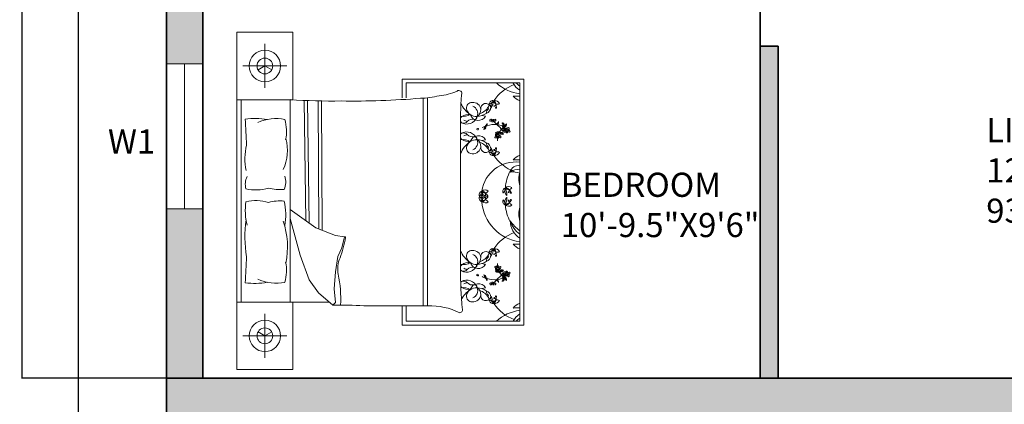
# Model space of a CAD drawing. Units: inches. Extents: x -9 to 505, y -680 to 48.
# Tile 3 of 17: x -9 to 235, y -293 to -198. Entities that reach past the tile are written whole.
import ezdxf

# ---------------------------------------------------------------- set-up
doc = ezdxf.new("R2010")
doc.units = ezdxf.units.IN
doc.header["$MEASUREMENT"] = 0
for name, color, linetype, lineweight in [('A-ANNO-DIMS', 2, 'Continuous', 18), ('A-ANNO-TEXT', 7, 'Continuous', 18), ('A-AREA-IDEN', 7, 'Continuous', 18), ('A-FURN', 8, 'Continuous', 18), ('A-GLAZ', 4, 'Continuous', 18), ('A-WALL', 7, 'Continuous', 35), ('A-WALL-PATT', 251, 'Continuous', 13), ('S-CONC', 7, 'Continuous', 35), ('S-CONC-PATT', 18, 'Continuous', 13)]:
    doc.layers.add(name, color=color, linetype=linetype, lineweight=lineweight)
doc.styles.get("Standard").update_dxf_attribs({"font": 'arial.ttf'})
doc.dimstyles.get("Standard").update_dxf_attribs({"dimtxt": 0.18, "dimasz": 0.18, "dimexe": 0.18, "dimexo": 0.0625, "dimgap": 0.09, "dimtad": 0, "dimtih": 1, "dimtoh": 1, "dimdec": 0, "dimzin": 0, "dimdsep": 46, "dimlunit": 3, "dimtxsty": 'Standard', "dimcen": 0.09, "dimadec": 0, "dimazin": 0, "dimtfac": 1, "dimtdec": 0, "dimtofl": 0, "dimtmove": 0, "dimatfit": 3, "dimfxl": 1, "dimtolj": 1, "dimtzin": 0, "dimarcsym": 0})

# ---------------------------------------------------------------- blocks, each defined once
blk = doc.blocks.new('*D3')
at = {"layer": 'A-ANNO-DIMS', "color": 0, "lineweight": -2, "transparency": 16777216}
for p, q in [((27.2, 11.5), (5.16, 11.5)), ((5.34, 11.32), (5.34, -330.86)), ((5.34, -679.32), (5.34, -337.14)), ((27.2, -679.5), (5.16, -679.5))]:
    blk.add_line(p, q, dxfattribs=at)
at = {"layer": 'A-ANNO-DIMS', "color": 0, "transparency": 16777216}
for points in [[(5.31, 11.32), (5.37, 11.32), (5.34, 11.5)], [(5.31, -679.32), (5.37, -679.32), (5.34, -679.5)]]:
    blk.add_solid(points, dxfattribs=at)
at = {"layer": 'Defpoints', "color": 0, "transparency": 16777216}
for p in [(27.26, 11.5), (5.34, -679.5), (27.26, -679.5)]:
    blk.add_point(p, dxfattribs=at)
at = {"layer": 'A-ANNO-DIMS', "color": 0, "transparency": 16777216, "insert": (5.34, -334), "char_height": 6, "attachment_point": 5}
blk.add_mtext('\\A1;57\'-7"', dxfattribs=at)
blk = doc.blocks.new('WIN-36')
for p, q in [((0, 36), (0, 0)), ((9, 36), (0, 36)), ((4.5, 36), (4.5, 2.23)), ((9, 0), (9, 36)), ((0, 0), (9, 0)), ((4.5, 2.23), (4.5, 0))]:
    blk.add_line(p, q)
blk = doc.blocks.new('*D46')
at = {"layer": 'A-ANNO-DIMS', "color": 0, "lineweight": -2, "transparency": 16777216}
for p, q in [((27.2, 11.5), (-8.8, 11.5)), ((-8.62, 11.32), (-8.62, -137.57)), ((-8.62, -286.82), (-8.62, -137.93)), ((27.2, -287), (-8.8, -287))]:
    blk.add_line(p, q, dxfattribs=at)
at = {"layer": 'A-ANNO-DIMS', "color": 0, "transparency": 16777216}
for points in [[(-8.65, 11.32), (-8.59, 11.32), (-8.62, 11.5)], [(-8.65, -286.82), (-8.59, -286.82), (-8.62, -287)]]:
    blk.add_solid(points, dxfattribs=at)
at = {"layer": 'Defpoints', "color": 0, "transparency": 16777216}
for p in [(27.26, 11.5), (-8.62, -287), (27.26, -287)]:
    blk.add_point(p, dxfattribs=at)
at = {"layer": 'A-ANNO-DIMS', "color": 0, "transparency": 16777216, "insert": (-8.62, -137.75), "char_height": 0.18, "attachment_point": 5}
blk.add_mtext('\\A1;24\'-10 1/2"', dxfattribs=at)

msp = doc.modelspace()

# ---------------------------------------------------------------- hatches: boundary and pattern name
at = {"layer": 'A-WALL-PATT'}
h = msp.add_hatch(color=256, dxfattribs=at)
h.dxf.hatch_style = 1
h.paths.add_polyline_path([(101.64, 11.5), (48.26, 11.5), (48.26, 2.5), (72.26, 2.5), (72.26, -21.25), (81.26, -21.25), (81.26, 2.5), (101.64, 2.5)])
h.paths.add_polyline_path([(36.26, 2.5), (27.26, 2.5), (27.26, -6.92), (36.26, -6.92)])
h.paths.add_polyline_path([(81.26, -57.25), (72.26, -57.25), (72.26, -75.5), (81.26, -75.5)])
h.paths.add_polyline_path([(162.76, 11.5), (137.64, 11.5), (137.64, 2.5), (162.76, 2.5)])
h.paths.add_polyline_path([(179.26, 2.5), (174.76, 2.5), (174.76, -75.5), (179.26, -75.5), (179.26, -54.5), (229.51, -54.5), (229.51, -45.5), (179.26, -45.5)])
h.paths.add_polyline_path([(382.26, -45.5), (332.26, -45.5), (332.26, 2.5), (327.76, 2.5), (327.76, -45.5), (277.51, -45.5), (277.51, -54.5), (327.76, -54.5), (327.76, -111.5), (332.26, -111.5), (332.26, -54.5), (382.26, -54.5)])
h.paths.add_polyline_path([(332.26, -128), (327.76, -128), (327.76, -207), (332.26, -207)])
h.paths.add_polyline_path([(124.76, -111.5), (36.26, -111.5), (36.26, -116), (120.26, -116), (120.26, -168.5), (179.26, -168.5), (179.26, -164), (124.76, -164)])
h.paths.add_polyline_path([(96.26, -164), (36.26, -164), (36.26, -152), (27.26, -152), (27.26, -208.88), (36.26, -208.88), (36.26, -168.5), (96.26, -168.5)])
h.paths.add_polyline_path([(36.26, -244.88), (27.26, -244.88), (27.26, -287), (36.26, -287)])
h.paths.add_polyline_path([(179.26, -204.5), (174.76, -204.5), (174.76, -287), (179.26, -287)])
h.paths.add_polyline_path([(257.26, -296), (248.26, -296), (248.26, -446), (269.26, -446), (269.26, -437), (257.26, -437)])
h.paths.add_polyline_path([(90.26, -296), (81.26, -296), (81.26, -348.67), (90.26, -348.67)])
h.paths.add_polyline_path([(90.26, -384.67), (81.26, -384.67), (81.26, -416), (90.26, -416)])
h.paths.add_polyline_path([(170.26, -452), (36.26, -452), (36.26, -456.5), (165.76, -456.5), (165.76, -504.5), (165.13, -504.5), (165.13, -509), (170.26, -509)])
h.paths.add_polyline_path([(141.76, -504.5), (36.26, -504.5), (36.26, -492.5), (27.26, -492.5), (27.26, -565.96), (36.26, -565.96), (36.26, -509), (141.76, -509)])
h.paths.add_polyline_path([(36.26, -601.96), (27.26, -601.96), (27.26, -658.5), (36.26, -658.5)])
h.paths.add_polyline_path([(170.26, -670.5), (170.26, -634.5), (222.76, -634.5), (222.76, -625.5), (165.76, -625.5), (165.76, -670.5), (36.26, -670.5), (36.26, -679.5), (170.26, -679.5)])
h.paths.add_polyline_path([(332.26, -616.5), (433.89, -616.5), (433.89, -612), (332.26, -612), (332.26, -610.56), (327.76, -610.56), (327.76, -625.5), (270.76, -625.5), (270.76, -634.5), (327.76, -634.5), (327.76, -658.5), (332.26, -658.5)])
h.paths.add_polyline_path([(459.76, -670.5), (336.76, -670.5), (336.76, -679.5), (459.76, -679.5)])
h.paths.add_polyline_path([(468.76, -545.74), (459.76, -545.74), (459.76, -612), (457.89, -612), (457.89, -616.5), (459.76, -616.5), (459.76, -658.5), (468.76, -658.5)])
h.paths.add_polyline_path([(332.26, -446), (327.76, -446), (327.76, -574.56), (332.26, -574.56)])
h.paths.add_polyline_path([(327.76, -437), (305.26, -437), (305.26, -446), (327.76, -446)])
h.paths.add_polyline_path([(459.76, -437), (348.76, -437), (348.76, -446), (459.76, -446)])
h.paths.add_polyline_path([(468.76, -458), (459.76, -458), (459.76, -509.74), (468.76, -509.74)])
h.paths.add_polyline_path([(468.76, -365), (459.76, -365), (459.76, -437), (468.76, -437)])
h.paths.add_polyline_path([(468.76, -299.6), (459.76, -299.6), (459.76, -344), (468.76, -344)])
h.paths.add_polyline_path([(468.76, -184.74), (459.76, -184.74), (459.76, -231), (401.26, -231), (401.26, -235.5), (459.76, -235.5), (459.76, -275.6), (468.76, -275.6)])
h.paths.add_polyline_path([(390.76, -356), (342.76, -356), (342.76, -365), (390.76, -365)])
h.paths.add_polyline_path([(459.76, -356), (405.76, -356), (405.76, -365), (459.76, -365)])
h.paths.add_polyline_path([(405.76, -296), (396.76, -296), (396.76, -356), (405.76, -356)])
h.paths.add_polyline_path([(336.76, -296), (327.76, -296), (327.76, -356), (336.76, -356)])
h.paths.add_polyline_path([(468.76, -9.5), (459.76, -9.5), (459.76, -45.5), (418.26, -45.5), (418.26, -54.5), (468.76, -54.5)])
h.paths.add_polyline_path([(468.76, -54.5), (459.76, -54.5), (459.76, -111.5), (468.76, -111.5)])
h.paths.add_polyline_path([(468.76, -128), (459.76, -128), (459.76, -148.74), (468.76, -148.74)])
at = {"layer": 'S-CONC-PATT'}
h = msp.add_hatch(color=256, dxfattribs=at)
h.dxf.hatch_style = 1
h.paths.add_polyline_path([(269.26, -296), (269.26, -287), (27.26, -287), (27.26, -308), (36.26, -308), (36.26, -296)])

# ---------------------------------------------------------------- linework, layer by layer
at = {"layer": 'A-FURN'}
for p, q in [((44.71, -284.86), (44.71, -201.01)), ((51.7, -214.87), (51.7, -203.92)), ((57.17, -209.4), (46.22, -209.4)), ((85.81, -217.31), (85.81, -212.66)), ((85.81, -212.66), (116.01, -212.66)), ((116.01, -212.66), (116.01, -273.79)), ((86.78, -213.63), (86.78, -217.33)), ((115.04, -213.63), (86.78, -213.63)), ((115.04, -272.82), (115.04, -213.63)), ((91.04, -217.4), (91.04, -269.05)), ((92.08, -217.32), (92.08, -269.05)), ((45.78, -217.78), (45.78, -268.09)), ((57.96, -268.09), (57.96, -217.78)), ((61.44, -218.01), (61.86, -247.86)), ((62.3, -218.04), (62.73, -248.48)), ((64.94, -218.08), (65.07, -249.92)), ((65.8, -218.08), (65.93, -250.25)), ((106.54, -221.9), (105.59, -221.71)), ((100.32, -225.91), (100.32, -259.95)), ((106.54, -227.76), (105.59, -227.94)), ((57.96, -245.05), (64.35, -249.65)), ((60.45, -256.44), (57.96, -247.3)), ((64.35, -249.65), (69.28, -251.52)), ((69.28, -251.52), (71.48, -251.86)), ((71.48, -251.86), (70.8, -254.57)), ((62.66, -262.55), (60.45, -256.44)), ((69.78, -256.78), (69.28, -260.52)), ((70.8, -254.57), (69.78, -256.78)), ((106.54, -258.7), (105.59, -258.51)), ((69.28, -260.52), (68.94, -264.76)), ((65.03, -265.78), (62.66, -262.55)), ((68.6, -268.84), (65.03, -265.78)), ((68.94, -264.76), (69.28, -268.16)), ((106.54, -264.56), (105.59, -264.74)), ((44.71, -268.09), (67.72, -268.09)), ((69.28, -268.16), (68.6, -268.84)), ((85.81, -273.79), (85.81, -269.05)), ((86.78, -269.05), (86.78, -272.82)), ((51.7, -270.99), (51.7, -281.95)), ((116.01, -273.79), (85.81, -273.79)), ((86.78, -272.82), (115.04, -272.82)), ((57.17, -276.47), (46.22, -276.47))]:
    msp.add_line(p, q, dxfattribs=at)
for points in [[(44.71, -217.78), (58.68, -217.78), (58.68, -201.01), (44.71, -201.01)], [(51.7, -209.4), (50, -210.37)], [(51.7, -209.4), (53.39, -210.37)], [(58.68, -268.09), (58.68, -284.86), (44.71, -284.86)], [(51.7, -276.47), (50, -275.49)], [(51.7, -276.47), (53.39, -275.49)]]:
    msp.add_lwpolyline(points, dxfattribs=at)
for points in [[(90.38, -217.42, 0.056112), (94.99, -216.81, 0.095341), (99.43, -215.64)], [(46.8, -222.6, -0.074897), (52.27, -222.7, 0.472817)], [(52.58, -239.75, -0.14099), (46.99, -239.91, -0.235245)], [(52.58, -243.33, 0.14099), (46.99, -243.16, 0.235245)], [(46.8, -263.27, 0.074897), (52.27, -263.17, -0.472817)], [(76.27, -269.01, 0.001242), (92.18, -269.05, -0.127202), (100.11, -270.73)]]:
    msp.add_lwpolyline(points, format="xyb", dxfattribs=at)
for centre, radius in [((51.7, -209.4), 3.91), ((51.7, -209.4), 1.96), ((109.58, -226.74), 0.214), ((111.83, -225.34), 0.214), ((109.58, -259.71), 0.214), ((111.83, -261.11), 0.214), ((51.7, -276.47), 3.91), ((51.7, -276.47), 1.96)]:
    msp.add_circle(centre, radius, dxfattribs=at)
for centre, radius, start, end in [((117.6, -224.22), 10.95, 111.4092, 145.6135), ((116.52, -205.48), 10.95, 228.1144, 262.255), ((117.98, -210.98), 5.34, 209.8884, 236.5383), ((118.98, -209.06), 6.65, 223.5186, 233.6964), ((73.68, -21.61), 196.52, 269.1145, 274.8735), ((99.86, -216.27), 0.764, 336.5219, 123.8264), ((181.87, -223.34), 81.59, 175.2402, 181.8035), ((116.75, -213.96), 4.45, 221.0454, 247.4453), ((114.36, -201.77), 15.15, 266.3481, 272.5919), ((68.2, -67.47), 150.65, 266.1, 270.9282), ((106.22, -216.16), 6.35, 203.6453, 236.3329), ((103.18, -219.86), 1.42, 88.9462, 185.5144), ((104.22, -219.43), 2.52, 193.079, 274.7067), ((103.38, -220.44), 2, 7.1143, 95.0551), ((102.62, -221.23), 1.95, 338.5779, 68.4181), ((103.84, -217.48), 3.96, 288.2955, 328.7386), ((106.61, -219.98), 1.26, 19.1312, 189.736), ((106.23, -219.68), 1.57, 285.6955, 4.031), ((108.32, -221.37), 1.67, 128.4175, 173.8338), ((107.97, -219.72), 0.771, 126.7319, 206.0245), ((108.35, -218.91), 0.908, 76.272, 177.0484), ((106.97, -217.06), 1.87, 284.7031, 328.6173), ((109.57, -219.44), 1.73, 125.7657, 194.5347), ((101.09, -216.37), 7.66, 332.8176, 347.4827), ((108.82, -219.22), 1.21, 20.9613, 102.2885), ((109.48, -218), 0.914, 181.7131, 301.5367), ((106.48, -219.85), 2.77, 2.0648, 41.1598), ((108.15, -218.82), 0.896, 316.2238, 62.3173), ((108.66, -219.35), 0.0714, 20.2667, 316.2271), ((109.11, -219.76), 0.136, 168.5166, 2.0648), ((109.04, -219.75), 0.0661, 52.0591, 168.5166), ((-751.12, -268.81), 799.26, 2.85022, 3.31479), ((54.47, -233.28), 10.81, 78.2417, 114.8684), ((101.25, -222.79), 1.01, 127.675, 162.5814), ((100.94, -218.49), 3.47, 259.249, 301.1782), ((101.84, -221.18), 2.67, 240.8249, 340.7178), ((102.45, -224.67), 3.23, 85.2696, 124.215), ((103.27, -224.34), 1.72, 74.8529, 138.4347), ((104.73, -220.86), 2.08, 196.8663, 330.0915), ((103.86, -222.18), 0.52, 254.8529, 12.6959), ((102.45, -224.67), 3.23, 53.6555, 57.2989), ((102.93, -220.09), 2.44, 305.9599, 357.6409), ((104.16, -217.45), 4.5, 273.4924, 303.7117), ((107.98, -222.9), 0.356, 127.3642, 168.4363), ((108.31, -222.6), 0.214, 183.2768, 356.7232), ((108.7, -222.89), 0.353, 10.9597, 52.2379), ((45.82, -225.59), 11.24, 348.9631, 14.8961), ((101.25, -222.79), 1.01, 196.6343, 225.5483), ((101.05, -222.37), 1.25, 246.1646, 318.4347), ((102.33, -220.78), 2.41, 240.0851, 262.564), ((104.55, -225.05), 0.263, 169.5864, 349.5616), ((104.65, -225.07), 0.162, 349.5616, 167.2949), ((108.87, -230.88), 6.94, 110.1059, 116.9968), ((105.27, -224.14), 1.33, 308.4388, 328.836), ((106.54, -225.16), 0.44, 129.5056, 182.6421), ((105.04, -223.06), 2.36, 296.5064, 305.3102), ((105.02, -224.28), 1.35, 336.3901, 344.4871), ((106.49, -224.62), 0.171, 83.9457, 185.6216), ((105.81, -224.46), 0.703, 328.836, 0.8141), ((106.17, -224.67), 0.402, 306.5232, 32.4668), ((106.65, -224.35), 0.171, 112.5583, 214.2343), ((106.54, -224.05), 0.402, 265.7131, 351.6568), ((106.19, -223.83), 0.703, 297.3659, 329.344), ((105.65, -223.22), 1.35, 313.6929, 321.7899), ((107.14, -224.14), 0.44, 115.5379, 168.6744), ((105.65, -223.51), 1.33, 329.344, 349.7412), ((108.87, -230.88), 6.94, 86.1723, 106.4158), ((104.59, -223.81), 2.36, 352.8698, 1.6736), ((107.72, -222.96), 0.165, 125.0752, 284.7644), ((107.7, -222.61), 0.513, 277.4968, 341.2737), ((108.11, -222.85), 0.204, 88.1325, 178.8919), ((108.52, -223.07), 0.441, 136.3462, 189.6513), ((108.26, -223.11), 0.184, 189.6513, 312.3208), ((108.98, -222.98), 0.699, 164.2829, 186.9148), ((108.15, -222.99), 0.349, 312.3208, 40.2111), ((108.89, -222.59), 0.496, 201.6382, 274.947), ((108.24, -223.27), 0.648, 42.3896, 66.5724), ((114.78, -218.14), 7.96, 217.9541, 226.8459), ((108.92, -222.93), 0.164, 274.947, 37.5263), ((109.47, -223.85), 0.171, 112.5583, 214.2343), ((109.36, -223.55), 0.402, 265.7131, 351.6568), ((109.01, -223.33), 0.703, 297.3659, 329.344), ((109.04, -227.42), 3.48, 60.7959, 85.244), ((101.63, -232.43), 11.46, 37.8256, 47.7588), ((108.48, -222.72), 1.35, 313.6929, 321.7899), ((109.97, -223.64), 0.44, 115.5379, 168.6744), ((108.47, -223.01), 1.33, 329.344, 349.7412), ((107.41, -223.31), 2.36, 352.8698, 1.6736), ((113.67, -227.78), 4.18, 130.182, 149.456), ((110.74, -223.79), 0.238, 33.0979, 123.1364), ((105.49, -227.15), 6.24, 31.1156, 34.8118), ((110.39, -224.2), 0.645, 2.3172, 70.5201), ((111.37, -225.4), 0.689, 139.3812, 199.9959), ((110.08, -224.9), 0.973, 310.9365, 22.7695), ((110.93, -224.36), 0.186, 135.7354, 318.1297), ((110.61, -224.06), 0.247, 315.7354, 31.1156), ((110.41, -224.58), 0.573, 319.3812, 5.5456), ((111.06, -224.36), 0.186, 68.2452, 250.6395), ((110.64, -224.13), 0.556, 352.6008, 57.1845), ((112.62, -227.86), 3.72, 111.7087, 116.2181), ((109.04, -227.42), 3.48, 47.5083, 55.9967), ((111.17, -224), 0.556, 252.8042, 349.6943), ((110.64, -225), 0.592, 331.1838, 51.6792), ((111.23, -223.96), 0.247, 248.2452, 323.6254), ((111.45, -225.08), 0.209, 138.2946, 276.2474), ((111.01, -223.8), 0.645, 291.7087, 3.0299), ((111.53, -225.11), 0.291, 358.5719, 143.8954), ((106.4, -220.4), 6.24, 323.6254, 327.3216), ((111.7, -224.88), 0.294, 208.8493, 269.9355), ((111.52, -223.97), 0.238, 325.6077, 55.6462), ((112.47, -225.29), 0.673, 121.9501, 165.2442), ((112.01, -225.03), 0.141, 262.868, 7.094), ((111.99, -224.91), 0.421, 278.5614, 22.5914), ((112.23, -224.9), 0.212, 44.3732, 121.9501), ((46.64, -230.44), 10.67, 333.8761, 16.1746), ((101.25, -226.86), 1.01, 134.4517, 156.7144), ((101.25, -226.86), 1.01, 203.2856, 232.325), ((101.84, -228.47), 2.67, 19.2822, 119.1751), ((101.05, -227.29), 1.25, 41.5653, 113.8354), ((102.33, -228.88), 2.41, 97.436, 119.9149), ((103.27, -225.31), 1.72, 221.5653, 285.1471), ((104.73, -228.8), 2.08, 29.9085, 163.1337), ((103.86, -227.48), 0.52, 347.3041, 105.1471), ((108.99, -227.1), 0.165, 125.0752, 284.7644), ((109.25, -227.04), 0.356, 93.635, 168.4363), ((109.26, -225.11), 0.973, 253.6301, 325.4631), ((109.53, -226.46), 0.689, 82.0748, 142.6895), ((109.46, -225.51), 0.707, 228.342, 274.9894), ((109.2, -226.47), 0.209, 138.2946, 276.2474), ((108.97, -226.75), 0.513, 277.4968, 341.2737), ((109.28, -226.51), 0.291, 358.5719, 143.8954), ((109.38, -226.99), 0.204, 88.1325, 178.8919), ((109.45, -226.28), 0.294, 208.8493, 269.9355), ((109.2, -226.35), 0.336, 274.2123, 318.1587), ((109.79, -227.21), 0.441, 136.3462, 189.6513), ((109.53, -227.25), 0.184, 189.6513, 312.3208), ((113.67, -227.78), 4.18, 175.2415, 182.8929), ((109.48, -225.63), 0.592, 273.8774, 357.1501), ((110.25, -227.12), 0.699, 164.2829, 186.9148), ((110.22, -226.68), 0.673, 121.9501, 165.2442), ((109.71, -225.21), 0.573, 262.0748, 308.2393), ((109.42, -227.13), 0.349, 312.3208, 40.2111), ((110.16, -226.73), 0.496, 201.6382, 274.947), ((109.76, -226.42), 0.141, 262.868, 7.094), ((109.5, -227.41), 0.648, 42.3896, 66.5724), ((109.74, -226.31), 0.421, 278.5614, 22.5914), ((109.97, -227.03), 0.353, 10.9597, 118.7804), ((113.67, -227.78), 4.18, 156.1523, 156.9499), ((109.98, -226.29), 0.212, 44.3732, 121.9501), ((110.63, -225.79), 0.592, 181.4625, 249.4747), ((110.53, -225.33), 0.573, 215.1128, 261.2773), ((110.99, -225.36), 0.973, 197.889, 269.722), ((110.19, -227.06), 0.164, 274.947, 37.5263), ((110.69, -225.69), 0.707, 248.3627, 295.0101), ((110.34, -226.58), 0.689, 20.6625, 81.2773), ((110.53, -224.95), 0.707, 285.6484, 332.2957), ((111.24, -225.7), 0.165, 125.0752, 284.7644), ((111.5, -225.64), 0.356, 93.635, 168.4363), ((111.22, -225.35), 0.513, 277.4968, 341.2737), ((111.63, -225.59), 0.204, 88.1325, 178.8919), ((111.45, -224.95), 0.336, 274.2123, 318.1587), ((112.04, -225.81), 0.441, 136.3462, 189.6513), ((111.78, -225.85), 0.184, 189.6513, 312.3208), ((112.5, -225.73), 0.699, 164.2829, 186.9148), ((111.67, -225.73), 0.349, 312.3208, 40.2111), ((112.41, -225.34), 0.496, 201.6382, 274.947), ((111.75, -226.02), 0.648, 42.3896, 66.5724), ((112.22, -225.64), 0.353, 10.9597, 118.7804), ((112.44, -225.67), 0.164, 274.947, 37.5263), ((61.47, -232.55), 14.74, 166.3427, 191.1841), ((100.94, -231.16), 3.47, 58.8218, 100.2867), ((106.22, -233.49), 6.35, 123.6671, 158.5059), ((102.45, -224.99), 3.23, 235.785, 274.7304), ((103.18, -229.79), 1.42, 174.4856, 271.0538), ((104.22, -230.23), 2.52, 85.2933, 166.921), ((103.38, -229.21), 2, 264.9449, 352.8857), ((102.62, -228.43), 1.95, 291.5819, 21.4221), ((102.45, -224.99), 3.23, 302.7011, 306.3445), ((102.93, -229.56), 2.44, 2.3591, 54.0401), ((104.16, -232.21), 4.5, 56.2883, 86.5076), ((103.84, -232.17), 3.96, 31.2614, 71.7045), ((106.61, -229.67), 1.26, 170.264, 340.8688), ((108.32, -228.28), 1.67, 186.1662, 231.5825), ((106.23, -229.98), 1.57, 355.969, 74.3045), ((107.97, -229.93), 0.771, 153.9755, 233.2681), ((109.57, -230.22), 1.73, 165.4653, 234.2343), ((101.09, -233.28), 7.66, 12.5173, 27.1824), ((106.48, -229.8), 2.77, 318.8402, 357.9352), ((109.11, -229.89), 0.136, 357.9352, 191.4834), ((109.04, -229.91), 0.0661, 191.4834, 307.9409), ((108.35, -230.74), 0.908, 182.9516, 283.728), ((106.97, -232.6), 1.87, 31.3827, 75.2969), ((108.15, -230.83), 0.896, 297.6827, 43.7762), ((109.48, -231.65), 0.914, 58.4633, 178.2869), ((108.82, -230.44), 1.21, 257.7115, 339.0387), ((117.6, -225.44), 10.95, 214.3865, 248.5908), ((108.71, -230.29), 0.118, 43.7762, 339.7183), ((116.75, -235.69), 4.45, 112.5547, 138.9546), ((113.99, -241.73), 8.47, 82.8636, 171.8197), ((114.58, -236.14), 1.97, 76.3898, 169.0739), ((114.36, -247.88), 15.15, 87.4081, 93.6519), ((50.98, -238.76), 4.15, 153.3437, 196.1026), ((52.43, -238.2), 4.44, 335.0183, 18.5407), ((122.38, -240.54), 10.95, 152.5854, 175.5377), ((114.31, -237.61), 2.49, 72.8609, 131.9049), ((113.21, -240.63), 4.9, 68.117, 96.6195), ((120.8, -237.48), 6.02, 162.9798, 196.4569), ((55.38, -229.86), 10.27, 254.1707, 275.9871), ((111.72, -240.56), 0.908, 106.1963, 206.9726), ((109.6, -239.64), 1.87, 314.6273, 358.5415), ((113.04, -240.4), 1.73, 155.6899, 224.4589), ((112.28, -240.58), 1.21, 50.8855, 132.2127), ((112.24, -239.21), 0.914, 211.6373, 331.4609), ((111.5, -240.58), 0.896, 346.148, 92.2415), ((110.57, -242.3), 2.77, 31.989, 71.0841), ((104.16, -241.98), 7.66, 2.7418, 17.407), ((123.9, -239.86), 8.9, 174.3643, 175.6213), ((130, -244.55), 15.91, 160.0972, 160.2783), ((105.85, -241.4), 0.908, 106.1963, 206.9726), ((105.85, -242.26), 0.908, 153.0274, 253.8037), ((103.73, -240.48), 1.87, 314.6273, 358.5415), ((103.73, -243.18), 1.87, 1.4585, 45.3727), ((107.18, -241.24), 1.73, 155.6899, 224.4589), ((107.18, -242.42), 1.73, 135.5411, 204.3101), ((106.42, -241.42), 1.21, 50.8855, 132.2127), ((106.38, -240.04), 0.914, 211.6373, 331.4609), ((105.64, -241.42), 0.896, 346.148, 92.2415), ((104.7, -243.14), 2.77, 31.989, 71.0841), ((98.29, -242.82), 7.66, 2.7418, 17.407), ((98.29, -240.84), 7.66, 342.593, 357.2582), ((104.7, -240.51), 2.77, 288.9159, 328.011), ((105.64, -242.24), 0.896, 267.7585, 13.852), ((106.34, -241.62), 0.0714, 50.1909, 346.0209), ((106.39, -242.05), 0.118, 13.852, 309.9245), ((106.87, -241.77), 0.0661, 81.9833, 198.4408), ((106.87, -241.89), 0.0661, 161.5592, 278.0167), ((106.94, -241.75), 0.136, 198.4408, 31.989), ((106.94, -241.91), 0.136, 328.011, 161.5592), ((113.04, -243.26), 1.73, 135.5411, 204.3101), ((104.16, -241.68), 7.66, 342.593, 357.2582), ((112.21, -240.78), 0.0714, 50.1909, 346.0209), ((112.8, -240.91), 0.136, 198.4408, 31.989), ((112.73, -240.93), 0.0661, 81.9833, 198.4408), ((61.77, -245.36), 14.94, 171.5249, 193.96), ((55.38, -253.21), 10.27, 84.0129, 105.8293), ((42.08, -246.48), 14.79, 349.8617, 13.6238), ((106.38, -243.61), 0.914, 28.5391, 148.3627), ((106.42, -242.23), 1.21, 227.7873, 309.1145), ((116.52, -242.28), 10.95, 184.4623, 262.255), ((111.72, -243.1), 0.908, 153.0274, 253.8037), ((109.6, -244.02), 1.87, 1.4585, 45.3727), ((110.57, -241.35), 2.77, 288.9159, 328.011), ((111.5, -243.08), 0.896, 267.7585, 13.852), ((112.24, -244.45), 0.914, 28.5391, 148.3627), ((112.28, -243.07), 1.21, 227.7873, 309.1145), ((122.38, -243.12), 10.95, 184.4623, 207.4146), ((112.25, -242.89), 0.118, 13.852, 309.9245), ((112.8, -242.75), 0.136, 328.011, 161.5592), ((112.73, -242.73), 0.0661, 161.5592, 278.0167), ((120.8, -246.18), 6.02, 163.5431, 197.0202), ((123.9, -243.8), 8.9, 184.3787, 185.6357), ((130, -239.11), 15.91, 199.7217, 199.9028), ((77.14, -251.78), 30.41, 172.2196, 189.497), ((37.83, -254.37), 19.49, 348.0397, 19.2615), ((117.98, -247.77), 5.34, 181.272, 236.5383), ((120.85, -242.36), 9.89, 214.0123, 234.053), ((118.98, -245.85), 6.65, 197.8504, 233.6964), ((71.55, -252.05), 0.202, 358.8623, 109.7536), ((117.6, -261.01), 10.95, 111.4092, 145.6135), ((39.8, -246.03), 32.52, 340.1194, 349.3383), ((114.36, -238.57), 15.15, 266.3481, 272.5919), ((116.75, -250.76), 4.45, 221.0454, 247.4453), ((-751.12, -217.06), 799.26, 356.68521, 357.14978), ((106.22, -252.96), 6.35, 201.4941, 236.3329), ((103.18, -256.66), 1.42, 88.9462, 185.5144), ((104.22, -256.22), 2.52, 193.079, 274.7067), ((103.38, -257.24), 2, 7.1143, 95.0551), ((102.62, -258.03), 1.95, 338.5779, 68.4181), ((103.84, -254.28), 3.96, 288.2955, 328.7386), ((106.61, -256.78), 1.26, 19.1312, 189.736), ((106.23, -256.48), 1.57, 285.6955, 4.031), ((108.32, -258.17), 1.67, 128.4175, 173.8338), ((107.97, -256.52), 0.771, 126.7319, 206.0245), ((108.35, -255.71), 0.908, 76.272, 177.0484), ((106.97, -253.86), 1.87, 284.7031, 328.6173), ((109.57, -256.23), 1.73, 125.7657, 194.5347), ((101.09, -253.17), 7.66, 332.8176, 347.4827), ((108.82, -256.02), 1.21, 20.9613, 102.2885), ((108.15, -255.62), 0.896, 316.2238, 62.3173), ((106.48, -256.65), 2.77, 2.0648, 41.1598), ((109.48, -254.8), 0.914, 181.7131, 301.5367), ((108.66, -256.15), 0.0714, 20.2667, 316.2271), ((109.11, -256.56), 0.136, 168.5166, 2.0648), ((109.04, -256.54), 0.0661, 52.0591, 168.5166), ((45.82, -260.28), 11.24, 345.1039, 11.0369), ((76.62, -259.84), 6.83, 156.2616, 191.3392), ((100.94, -255.29), 3.47, 259.7133, 301.1782), ((101.25, -259.59), 1.01, 127.675, 156.7144), ((101.84, -257.98), 2.67, 240.8249, 340.7178), ((102.45, -261.47), 3.23, 85.2696, 124.215), ((104.73, -257.66), 2.08, 196.8663, 330.0915), ((103.86, -258.98), 0.52, 254.8529, 12.6959), ((102.45, -261.47), 3.23, 53.6555, 57.2989), ((102.93, -256.89), 2.44, 305.9599, 357.6409), ((104.16, -254.25), 4.5, 273.4924, 303.7117), ((108.99, -259.35), 0.165, 75.2356, 234.9248), ((108.97, -259.7), 0.513, 18.7263, 82.5032), ((109.79, -259.25), 0.441, 170.3487, 223.6538), ((109.53, -259.2), 0.184, 47.6792, 170.3487), ((113.67, -258.67), 4.18, 177.1071, 184.7585), ((110.25, -259.33), 0.699, 173.0852, 195.7171), ((109.42, -259.32), 0.349, 319.7889, 47.6792), ((110.16, -259.72), 0.496, 85.053, 158.3618), ((110.19, -259.39), 0.164, 322.4737, 85.053), ((38.9, -267.4), 31.64, 357.4519, 11.3392), ((187.6, -260.95), 87.28, 179.3433, 185.6887), ((101.25, -259.59), 1.01, 203.229, 225.5483), ((101.05, -259.16), 1.25, 246.1646, 318.4347), ((102.33, -257.58), 2.41, 240.0851, 262.564), ((103.27, -261.14), 1.72, 74.8529, 138.4347), ((104.55, -261.4), 0.263, 10.4384, 190.4136), ((104.65, -261.38), 0.162, 192.7051, 10.4384), ((108.87, -255.57), 6.94, 243.0032, 249.8941), ((105.27, -262.31), 1.33, 31.164, 51.5612), ((106.54, -261.3), 0.44, 177.3579, 230.4944), ((105.04, -263.39), 2.36, 54.6898, 63.4936), ((105.02, -262.18), 1.35, 15.5129, 23.6099), ((106.17, -261.79), 0.402, 327.5332, 53.4768), ((105.81, -261.99), 0.703, 359.1859, 31.164), ((109.25, -259.42), 0.356, 191.5637, 266.365), ((109.2, -259.98), 0.209, 83.7526, 221.7054), ((109.46, -260.94), 0.707, 85.0106, 131.658), ((109.26, -261.35), 0.973, 34.5369, 106.3699), ((109.53, -259.99), 0.689, 217.3105, 277.9252), ((109.28, -259.95), 0.291, 216.1046, 1.4281), ((109.38, -259.46), 0.204, 181.1081, 271.8675), ((109.45, -260.18), 0.294, 90.0645, 151.1507), ((109.2, -260.11), 0.336, 41.8413, 85.7877), ((101.63, -254.02), 11.46, 312.2412, 322.1744), ((109.48, -260.83), 0.592, 2.8499, 86.1226), ((110.22, -259.77), 0.673, 194.7558, 238.0499), ((109.71, -261.24), 0.573, 51.7607, 97.9252), ((109.76, -260.03), 0.141, 352.906, 97.132), ((109.5, -259.04), 0.648, 293.4276, 317.6104), ((109.97, -259.42), 0.353, 241.2196, 349.0403), ((109.74, -260.15), 0.421, 337.4086, 81.4386), ((113.67, -258.67), 4.18, 203.0501, 203.8477), ((109.98, -260.16), 0.212, 238.0499, 315.6268), ((110.63, -260.66), 0.592, 110.5253, 178.5375), ((110.99, -261.09), 0.973, 90.278, 162.111), ((110.53, -261.12), 0.573, 98.7227, 144.8872), ((113.67, -258.67), 4.18, 210.544, 229.818), ((110.69, -260.76), 0.707, 64.9899, 111.6373), ((110.34, -259.88), 0.689, 278.7227, 339.3375), ((111.37, -261.05), 0.689, 160.0041, 220.6188), ((110.08, -261.55), 0.973, 337.2305, 49.0635), ((110.53, -261.5), 0.707, 27.7043, 74.3516), ((110.41, -261.87), 0.573, 354.4544, 40.6188), ((109.04, -259.03), 3.48, 304.0033, 312.4917), ((110.64, -261.45), 0.592, 308.3208, 28.8162), ((111.24, -260.75), 0.165, 75.2356, 234.9248), ((111.5, -260.81), 0.356, 191.5637, 266.365), ((111.45, -261.38), 0.209, 83.7526, 221.7054), ((111.22, -261.1), 0.513, 18.7263, 82.5032), ((111.53, -261.34), 0.291, 216.1046, 1.4281), ((111.63, -260.86), 0.204, 181.1081, 271.8675), ((111.7, -261.57), 0.294, 90.0645, 151.1507), ((111.45, -261.5), 0.336, 41.8413, 85.7877), ((111.78, -260.6), 0.184, 47.6792, 170.3487), ((112.04, -260.64), 0.441, 170.3487, 223.6538), ((112.5, -260.73), 0.699, 173.0852, 195.7171), ((112.47, -261.16), 0.673, 194.7558, 238.0499), ((111.67, -260.72), 0.349, 319.7889, 47.6792), ((112.41, -261.12), 0.496, 85.053, 158.3618), ((112.01, -261.42), 0.141, 352.906, 97.132), ((111.75, -260.44), 0.648, 293.4276, 317.6104), ((112.22, -260.82), 0.353, 241.2196, 349.0403), ((111.99, -261.54), 0.421, 337.4086, 81.4386), ((112.23, -261.56), 0.212, 238.0499, 315.6268), ((112.44, -260.78), 0.164, 322.4737, 85.053), ((54.47, -252.59), 10.81, 245.1316, 281.7583), ((101.25, -263.66), 1.01, 134.4517, 153.558), ((101.25, -263.66), 1.01, 210.0293, 232.325), ((101.84, -265.27), 2.67, 19.2822, 119.1751), ((101.05, -264.09), 1.25, 41.5653, 113.8354), ((102.33, -265.67), 2.41, 97.436, 119.9149), ((103.27, -262.11), 1.72, 221.5653, 285.1471), ((104.73, -265.59), 2.08, 29.9085, 163.1337), ((103.86, -264.27), 0.52, 347.3041, 105.1471), ((106.49, -261.83), 0.171, 174.3784, 276.0543), ((106.65, -262.1), 0.171, 145.7657, 247.4417), ((106.54, -262.4), 0.402, 8.3432, 94.2869), ((106.19, -262.63), 0.703, 30.656, 62.6341), ((105.65, -263.23), 1.35, 38.2101, 46.3071), ((107.14, -262.31), 0.44, 191.3256, 244.4621), ((105.65, -262.94), 1.33, 10.2588, 30.656), ((108.87, -255.57), 6.94, 253.5842, 273.8277), ((104.59, -262.64), 2.36, 358.3264, 7.1302), ((107.72, -263.49), 0.165, 75.2356, 234.9248), ((107.98, -263.56), 0.356, 191.5637, 232.6358), ((107.7, -263.84), 0.513, 18.7263, 82.5032), ((108.11, -263.6), 0.204, 181.1081, 271.8675), ((108.26, -263.34), 0.184, 47.6792, 170.3487), ((108.52, -263.39), 0.441, 170.3487, 223.6538), ((108.31, -263.85), 0.214, 3.2768, 176.7232), ((108.98, -263.47), 0.699, 173.0852, 195.7171), ((108.15, -263.46), 0.349, 319.7889, 47.6792), ((108.89, -263.86), 0.496, 85.053, 158.3618), ((108.24, -263.18), 0.648, 293.4276, 317.6104), ((114.78, -268.31), 7.96, 133.1541, 142.0459), ((108.7, -263.56), 0.353, 307.7621, 349.0403), ((108.92, -263.53), 0.164, 322.4737, 85.053), ((109.47, -262.6), 0.171, 145.7657, 247.4417), ((109.04, -259.03), 3.48, 274.756, 299.2041), ((109.36, -262.9), 0.402, 8.3432, 94.2869), ((109.01, -263.13), 0.703, 30.656, 62.6341), ((108.48, -263.73), 1.35, 38.2101, 46.3071), ((109.97, -262.81), 0.44, 191.3256, 244.4621), ((108.47, -263.44), 1.33, 10.2588, 30.656), ((107.41, -263.14), 2.36, 358.3264, 7.1302), ((110.39, -262.25), 0.645, 289.4799, 357.6828), ((105.49, -259.3), 6.24, 325.1882, 328.8844), ((110.74, -262.66), 0.238, 236.8636, 326.9021), ((110.93, -262.09), 0.186, 41.8703, 224.2646), ((110.61, -262.4), 0.247, 328.8844, 44.2646), ((111.06, -262.09), 0.186, 109.3605, 291.7548), ((110.64, -262.32), 0.556, 302.8155, 7.3992), ((112.62, -258.59), 3.72, 243.7819, 248.2913), ((111.17, -262.45), 0.556, 10.3057, 107.1958), ((111.23, -262.5), 0.247, 36.3746, 111.7548), ((111.01, -262.65), 0.645, 356.9701, 68.2913), ((106.4, -266.05), 6.24, 32.6784, 36.3746), ((111.52, -262.48), 0.238, 304.3538, 34.3923), ((100.94, -267.96), 3.47, 58.8218, 99.1554), ((106.22, -270.29), 6.35, 123.6671, 153.2997), ((102.45, -261.78), 3.23, 235.785, 274.7304), ((103.18, -266.59), 1.42, 174.4856, 271.0538), ((104.22, -267.03), 2.52, 85.2933, 166.921), ((103.38, -266.01), 2, 264.9449, 352.8857), ((102.62, -265.22), 1.95, 291.5819, 21.4221), ((102.45, -261.78), 3.23, 302.7011, 306.3445), ((102.93, -266.36), 2.44, 2.3591, 54.0401), ((104.16, -269), 4.5, 56.2883, 86.5076), ((103.84, -268.97), 3.96, 31.2614, 71.7045), ((106.61, -266.47), 1.26, 170.264, 340.8688), ((106.23, -266.77), 1.57, 355.969, 74.3045), ((108.32, -265.08), 1.67, 186.1662, 231.5825), ((107.97, -266.73), 0.771, 153.9755, 233.2681), ((109.57, -267.02), 1.73, 165.4653, 234.2343), ((101.09, -270.08), 7.66, 12.5173, 27.1824), ((109.11, -266.69), 0.136, 357.9352, 191.4834), ((70.68, -345.71), 76.9, 85.8294, 91.553), ((106.97, -269.39), 1.87, 31.3827, 75.2969), ((108.35, -267.54), 0.908, 182.9516, 283.728), ((106.48, -266.6), 2.77, 318.8402, 357.9352), ((108.15, -267.63), 0.896, 297.6827, 43.7762), ((109.48, -268.45), 0.914, 58.4633, 178.2869), ((108.82, -267.23), 1.21, 257.7115, 339.0387), ((117.6, -262.24), 10.95, 214.3865, 248.5908), ((108.71, -267.09), 0.118, 43.7762, 339.7183), ((109.04, -266.71), 0.0661, 191.4834, 307.9409), ((116.75, -272.49), 4.45, 112.5547, 138.9546), ((100.06, -269.96), 0.774, 273.98, 27.3412), ((116.52, -280.97), 10.95, 97.745, 131.8856), ((117.98, -275.48), 5.34, 123.4617, 150.1116), ((114.36, -284.68), 15.15, 87.4081, 93.6519), ((118.98, -277.4), 6.65, 126.3036, 136.4814)]:
    msp.add_arc(centre, radius, start, end, dxfattribs=at)
at = {"layer": 'A-WALL'}
for p, q in [((27.26, 11.5), (27.26, -679.5)), ((36.26, -168.5), (36.26, -287)), ((174.76, -168.5), (174.76, -287)), ((179.26, -204.5), (174.76, -204.5)), ((179.26, -204.5), (179.26, -287))]:
    msp.add_line(p, q, dxfattribs=at)
at = {"layer": 'S-CONC'}
msp.add_line((27.26, -287), (269.26, -287), dxfattribs=at)

# ---------------------------------------------------------------- block references
at = {"layer": 'A-GLAZ'}
msp.add_blockref('WIN-36', (27.26, -244.88), dxfattribs=at)

# ---------------------------------------------------------------- texts
at = {"layer": 'A-ANNO-TEXT', "insert": (12.71, -225.18), "char_height": 6, "attachment_point": 1}
msp.add_mtext('W1', dxfattribs=at)
at = {"layer": 'A-AREA-IDEN', "char_height": 6, "attachment_point": 1}
for s, insert in [('LIVING\\P12\'0"X19\'4.5"\\P930.0 SQFT', (230.92, -222.36)), ('BEDROOM\\P10\'-9.5"X9\'6"', (125.2, -235.93))]:
    msp.add_mtext(s, dxfattribs=dict(at, insert=insert))

# ---------------------------------------------------------------- dimensions: what is measured, and where the dimension line sits
at = {"layer": 'A-ANNO-DIMS'}
for base, p2, override, picture, middle in [((-8.62, -287), (27.26, -287), {"dimdec": 1, "dimlfac": 1, "dimrnd": 0, "dimzin": 1, "dimdsep": 46, "dimlunit": 4, "dimfrac": 2}, '*D46', (-8.62, -137.75)), ((5.34, -679.5), (27.26, -679.5), {"dimtxt": 6, "dimclrd": 0, "dimclre": 0, "dimclrt": 0}, '*D3', (5.34, -334))]:
    dim = msp.add_linear_dim(base=base, p1=(27.26, 11.5), p2=p2, angle=90, dimstyle='Standard', override=override, dxfattribs=at)
    dim.commit()
    dim.dimension.update_dxf_attribs({"geometry": picture, "text_midpoint": middle})

doc.saveas('drawing.dxf')
